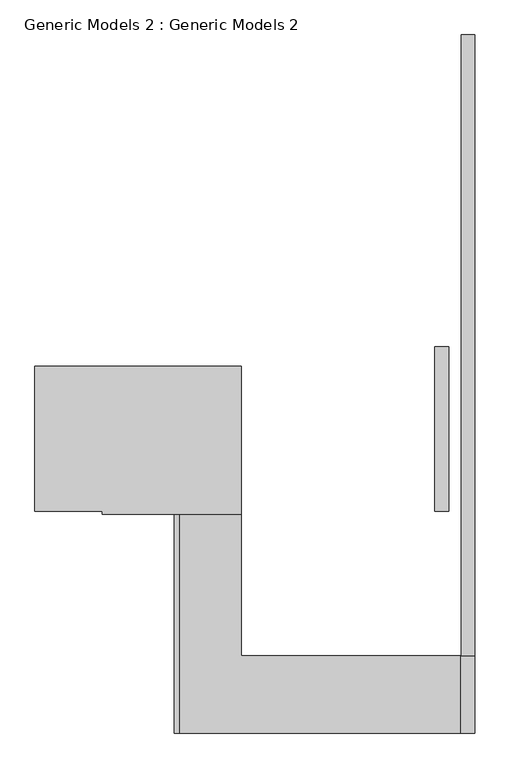
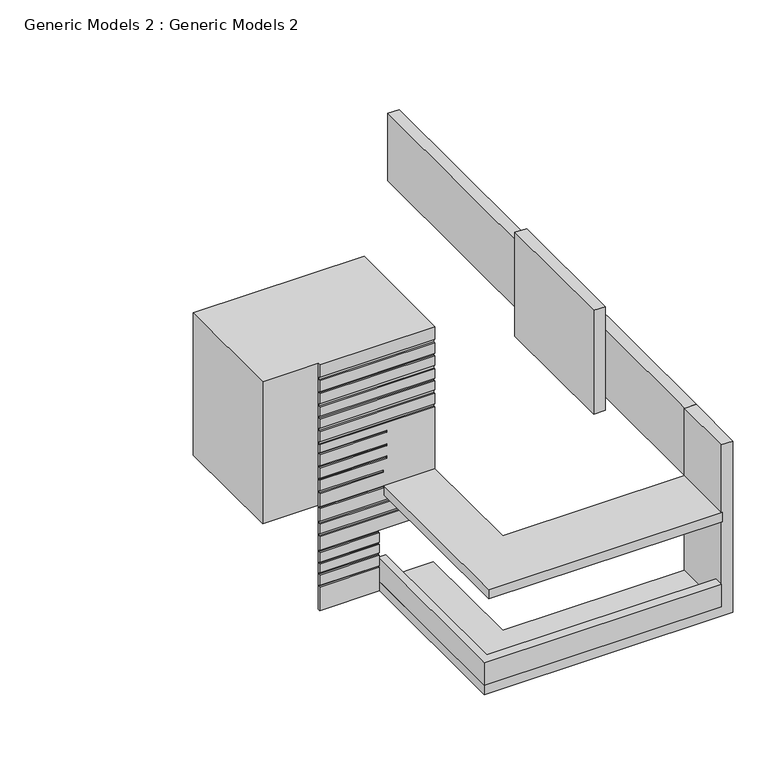
"""IFC4 building model written with IfcOpenShell, lengths in millimetres: proxy geometry, Generic Models 2 : Generic Models 2."""

from ifc_helpers import new_model, si_unit, frame, origin, place, context, project, spatial, polyline, outline, extrude, faceted_brep, source, transform, mapped, element, save


def generic_models_2_generic_models_2_8bbb9965(model_context):
    return source(origin(), model_context, "Body", "SolidModel", [
        extrude(outline(polyline([(-12215.152412, -15011.776778), (-12215.152412, -9476.6468404), (-10657.4321088, -9476.6468404), (-10657.4321088, -13058.0468404), (-5084.7494797, -13058.0468404), (-5084.7494797, -15011.776778), (-12215.152412, -15011.776778)])), frame((0.0, 0.0, 6096.0), z_axis=(0.0, 0.0, 1.0), x_axis=(1.0, 0.0, 0.0)), (0.0, 0.0, 1.0), 304.8),
        faceted_brep([(-15877.1321088, -9400.4468404, 6400.8), (-15877.1321088, -5738.2962979, 6400.8), (-10657.4321088, -5738.2962979, 6400.8), (-10657.4321088, -9400.4468404, 6400.8), (-14180.7645284, -9400.4468404, 6400.8), (-15877.1321088, -9400.4468404, 10988.8045332), (-14180.7645284, -9400.4468404, 10988.8045332), (-15877.1321088, -5738.2962979, 10988.8045332), (-10657.4321088, -5738.2962979, 10988.8045332), (-10657.4321088, -9476.6468404, 10988.8045332), (-14180.7645284, -9476.6468404, 10988.8045332), (-14180.7645284, -9476.6468404, 10585.2742098), (-10657.4321088, -9476.6468404, 10585.2742098), (-14180.7645284, -9476.6468404, 3048.0), (-12351.7136239, -9476.6468404, 3048.0), (-12351.7136239, -9476.6468404, 3808.1006121), (-14180.7645284, -9476.6468404, 3808.1006121), (-10657.4321088, -9476.6468404, 10470.2187496), (-14180.7645284, -9476.6468404, 10470.2187496), (-14180.7645284, -9476.6468404, 10122.5004137), (-10657.4321088, -9476.6468404, 10122.5004137), (-12351.7136239, -9476.6468404, 4611.1019692), (-12351.7136239, -9476.6468404, 4920.5427652), (-14180.7645284, -9476.6468404, 4920.5427652), (-14180.7645284, -9476.6468404, 4611.1019692), (-12351.7136239, -9476.6468404, 4276.4973082), (-12351.7136239, -9476.6468404, 4545.5762612), (-14180.7645284, -9476.6468404, 4545.5762612), (-14180.7645284, -9476.6468404, 4276.4973082), (-12351.7136239, -9476.6468404, 3862.9129914), (-12351.7136239, -9476.6468404, 4196.7702109), (-14180.7645284, -9476.6468404, 4196.7702109), (-14180.7645284, -9476.6468404, 3862.9129914), (-10657.4321088, -9476.6468404, 9733.5791761), (-10657.4321088, -9476.6468404, 10048.7503573), (-14180.7645284, -9476.6468404, 10048.7503573), (-14180.7645284, -9476.6468404, 9733.5791761), (-10657.4321088, -9476.6468404, 9327.208916), (-10657.4321088, -9476.6468404, 9618.9714739), (-14180.7645284, -9476.6468404, 9618.9714739), (-14180.7645284, -9476.6468404, 9327.208916), (-10657.4321088, -9476.6468404, 8943.2731135), (-10657.4321088, -9476.6468404, 9235.5227542), (-14180.7645284, -9476.6468404, 9235.5227542), (-14180.7645284, -9476.6468404, 8943.2731135), (-10657.4321088, -9476.6468404, 8496.3030748), (-10657.4321088, -9476.6468404, 8828.6654113), (-14180.7645284, -9476.6468404, 8828.6654113), (-14180.7645284, -9476.6468404, 8496.3030748), (-10657.4321088, -9476.6468404, 5929.0905449), (-10657.4321088, -9476.6468404, 8398.8865279), (-14180.7645284, -9476.6468404, 8398.8865279), (-14180.7645284, -9476.6468404, 8150.3954044), (-12128.9471301, -9476.6468404, 8150.3954044), (-12128.9471301, -9476.6468404, 8086.8954044), (-14180.7645284, -9476.6468404, 8086.8954044), (-14180.7645284, -9476.6468404, 7722.7010848), (-12128.9471301, -9476.6468404, 7722.7010848), (-12128.9471301, -9476.6468404, 7648.2060783), (-14180.7645284, -9476.6468404, 7648.2060783), (-14180.7645284, -9476.6468404, 7327.3045121), (-12128.9471301, -9476.6468404, 7327.3045121), (-12128.9471301, -9476.6468404, 7252.8095056), (-14180.7645284, -9476.6468404, 7252.8095056), (-14180.7645284, -9476.6468404, 6914.716784), (-12215.152412, -9476.6468404, 6914.716784), (-12215.152412, -9476.6468404, 6823.0306223), (-14180.7645284, -9476.6468404, 6823.0306223), (-14180.7645284, -9476.6468404, 6400.8), (-12215.152412, -9476.6468404, 6400.8), (-12215.152412, -9476.6468404, 6335.9478878), (-14180.7645284, -9476.6468404, 6335.9478878), (-14180.7645284, -9476.6468404, 5929.0905449), (-10657.4321088, -9476.6468404, 5527.9635871), (-10657.4321088, -9476.6468404, 5837.4043831), (-14180.7645284, -9476.6468404, 5837.4043831), (-14180.7645284, -9476.6468404, 5527.9635871), (-14180.7645284, -9476.6468404, 5004.8316632), (-10657.4321088, -9476.6468404, 5004.8316632), (-10657.4321088, -9476.6468404, 5430.5470402), (-14180.7645284, -9476.6468404, 5430.5470402), (-14180.7645284, -9400.4468404, 3048.0), (-14180.7645284, -9425.8468404, 3808.1006121), (-14180.7645284, -9425.8468404, 3862.9129914), (-14180.7645284, -9425.8468404, 4196.7702109), (-14180.7645284, -9425.8468404, 4276.4973082), (-14180.7645284, -9425.8468404, 4545.5762612), (-14180.7645284, -9425.8468404, 4611.1019692), (-14180.7645284, -9425.8468404, 4920.5427652), (-14180.7645284, -9425.8468404, 5004.8316632), (-14180.7645284, -9425.8468404, 5430.5470402), (-14180.7645284, -9425.8468404, 5527.9635871), (-14180.7645284, -9425.8468404, 5837.4043831), (-14180.7645284, -9425.8468404, 5929.0905449), (-14180.7645284, -9425.8468404, 6335.9478878), (-14180.7645284, -9425.8468404, 6400.8), (-14180.7645284, -9425.8468404, 6823.0306223), (-14180.7645284, -9425.8468404, 6914.716784), (-14180.7645284, -9425.8468404, 7252.8095056), (-14180.7645284, -9425.8468404, 7327.3045121), (-14180.7645284, -9425.8468404, 7648.2060783), (-14180.7645284, -9425.8468404, 7722.7010848), (-14180.7645284, -9425.8468404, 8086.8954044), (-14180.7645284, -9425.8468404, 8150.3954044), (-14180.7645284, -9425.8468404, 8398.8865279), (-14180.7645284, -9425.8468404, 8496.3030748), (-14180.7645284, -9425.8468404, 8828.6654113), (-14180.7645284, -9425.8468404, 8943.2731135), (-14180.7645284, -9425.8468404, 9235.5227542), (-14180.7645284, -9425.8468404, 9327.208916), (-14180.7645284, -9425.8468404, 9618.9714739), (-14180.7645284, -9425.8468404, 9733.5791761), (-14180.7645284, -9425.8468404, 10048.7503573), (-14180.7645284, -9425.8468404, 10122.5004137), (-14180.7645284, -9425.8468404, 10470.2187496), (-14180.7645284, -9425.8468404, 10585.2742098), (-10657.4321088, -9425.8468404, 10585.2742098), (-10657.4321088, -9425.8468404, 10470.2187496), (-10657.4321088, -9425.8468404, 10122.5004137), (-10657.4321088, -9425.8468404, 10048.7503573), (-10657.4321088, -9425.8468404, 9733.5791761), (-10657.4321088, -9425.8468404, 9618.9714739), (-10657.4321088, -9425.8468404, 9327.208916), (-10657.4321088, -9425.8468404, 9235.5227542), (-10657.4321088, -9425.8468404, 8943.2731135), (-10657.4321088, -9425.8468404, 8828.6654113), (-10657.4321088, -9425.8468404, 8496.3030748), (-10657.4321088, -9425.8468404, 8398.8865279), (-10657.4321088, -9425.8468404, 5929.0905449), (-10657.4321088, -9425.8468404, 5837.4043831), (-10657.4321088, -9425.8468404, 5527.9635871), (-10657.4321088, -9425.8468404, 5430.5470402), (-10657.4321088, -9400.4468404, 5004.8316632), (-12351.7136239, -9400.4468404, 5004.8316632), (-12351.7136239, -9400.4468404, 3048.0), (-12351.7136239, -9425.8468404, 5004.8316632), (-12351.7136239, -9425.8468404, 4920.5427652), (-12351.7136239, -9425.8468404, 4611.1019692), (-12351.7136239, -9425.8468404, 4545.5762612), (-12351.7136239, -9425.8468404, 4276.4973082), (-12351.7136239, -9425.8468404, 4196.7702109), (-12351.7136239, -9425.8468404, 3862.9129914), (-12351.7136239, -9425.8468404, 3808.1006121), (-12128.9471301, -9425.8468404, 8150.3954044), (-12128.9471301, -9425.8468404, 8086.8954044), (-12128.9471301, -9425.8468404, 7722.7010848), (-12128.9471301, -9425.8468404, 7648.2060783), (-12128.9471301, -9425.8468404, 7327.3045121), (-12128.9471301, -9425.8468404, 7252.8095056), (-12215.152412, -9425.8468404, 6914.716784), (-12215.152412, -9425.8468404, 6823.0306223), (-12215.152412, -9425.8468404, 6400.8), (-12215.152412, -9425.8468404, 6335.9478878)], [[[0, 1, 2, 3, 4]], [[5, 0, 4, 6]], [[7, 8, 2, 1]], [[5, 7, 1, 0]], [[9, 10, 11, 12]], [[13, 14, 15, 16]], [[17, 18, 19, 20]], [[21, 22, 23, 24]], [[25, 26, 27, 28]], [[29, 30, 31, 32]], [[33, 34, 35, 36]], [[37, 38, 39, 40]], [[41, 42, 43, 44]], [[45, 46, 47, 48]], [[49, 50, 51, 52, 53, 54, 55, 56, 57, 58, 59, 60, 61, 62, 63, 64, 65, 66, 67, 68, 69, 70, 71, 72]], [[73, 74, 75, 76]], [[77, 78, 79, 80]], [[10, 6, 4, 81, 13, 16, 82, 83, 32, 31, 84, 85, 28, 27, 86, 87, 24, 23, 88, 89, 77, 80, 90, 91, 76, 75, 92, 93, 72, 71, 94, 95, 68, 67, 96, 97, 64, 63, 98, 99, 60, 59, 100, 101, 56, 55, 102, 103, 52, 51, 104, 105, 48, 47, 106, 107, 44, 43, 108, 109, 40, 39, 110, 111, 36, 35, 112, 113, 19, 18, 114, 115, 11]], [[10, 9, 8, 7, 5, 6]], [[2, 8, 9, 12, 116, 117, 17, 20, 118, 119, 34, 33, 120, 121, 38, 37, 122, 123, 42, 41, 124, 125, 46, 45, 126, 127, 50, 49, 128, 129, 74, 73, 130, 131, 79, 78, 132, 3]], [[3, 132, 133, 134, 81, 4]], [[132, 78, 77, 89, 135, 133]], [[14, 13, 81, 134]], [[134, 133, 135, 136, 22, 21, 137, 138, 26, 25, 139, 140, 30, 29, 141, 142, 15, 14]], [[116, 115, 114, 117]], [[117, 114, 18, 17]], [[115, 116, 12, 11]], [[135, 89, 88, 136]], [[118, 113, 112, 119]], [[120, 111, 110, 121]], [[122, 109, 108, 123]], [[124, 107, 106, 125]], [[126, 105, 104, 127]], [[143, 103, 102, 144]], [[145, 101, 100, 146]], [[147, 99, 98, 148]], [[149, 97, 96, 150]], [[151, 95, 94, 152]], [[128, 93, 92, 129]], [[130, 91, 90, 131]], [[137, 87, 86, 138]], [[139, 85, 84, 140]], [[141, 83, 82, 142]], [[119, 112, 35, 34]], [[113, 118, 20, 19]], [[121, 110, 39, 38]], [[111, 120, 33, 36]], [[123, 108, 43, 42]], [[109, 122, 37, 40]], [[125, 106, 47, 46]], [[107, 124, 41, 44]], [[127, 104, 51, 50]], [[105, 126, 45, 48]], [[143, 144, 54, 53]], [[144, 102, 55, 54]], [[103, 143, 53, 52]], [[145, 146, 58, 57]], [[146, 100, 59, 58]], [[101, 145, 57, 56]], [[147, 148, 62, 61]], [[148, 98, 63, 62]], [[99, 147, 61, 60]], [[149, 150, 66, 65]], [[150, 96, 67, 66]], [[97, 149, 65, 64]], [[151, 152, 70, 69]], [[152, 94, 71, 70]], [[95, 151, 69, 68]], [[129, 92, 75, 74]], [[93, 128, 49, 72]], [[131, 90, 80, 79]], [[91, 130, 73, 76]], [[136, 88, 23, 22]], [[138, 86, 27, 26]], [[87, 137, 21, 24]], [[140, 84, 31, 30]], [[85, 139, 25, 28]], [[142, 82, 16, 15]], [[83, 141, 29, 32]]]),
        extrude(outline(polyline([(-5098.6527592, -13058.0468404), (-5098.6527592, 2639.1531596), (-4751.9321088, 2639.1531596), (-4751.9321088, -13058.0468404), (-5098.6527592, -13058.0468404)])), frame((0.0, 0.0, 6400.8), z_axis=(0.0, 0.0, 1.0), x_axis=(1.0, 0.0, 0.0)), (0.0, 0.0, 1.0), 2178.143726),
        extrude(outline(polyline([(-5417.9230491, -9400.4468404), (-5770.8398298, -9400.4468404), (-5770.8398298, -5247.5468404), (-5417.9230491, -5247.5468404), (-5417.9230491, -9400.4468404)])), frame((0.0, 0.0, 6400.8), z_axis=(0.0, 0.0, 1.0), x_axis=(1.0, 0.0, 0.0)), (0.0, 0.0, 1.0), 3351.6929741),
        extrude(outline(polyline([(-12351.7136239, -9400.4468404), (-12120.513383, -9400.4468404), (-12120.513383, -14738.7800298), (-5107.5321088, -14738.7800298), (-5107.5321088, -15011.776778), (-12351.7136239, -15011.776778), (-12351.7136239, -9400.4468404)])), frame((0.0, 0.0, 3352.8), z_axis=(0.0, 0.0, 1.0), x_axis=(1.0, 0.0, 0.0)), (0.0, 0.0, 1.0), 736.6),
        faceted_brep([(-12351.7136239, -15011.776778, 3048.0), (-12351.7136239, -15011.776778, 3352.8), (-12351.7136239, -9400.4468404, 3352.8), (-12351.7136239, -9400.4468404, 3048.0), (-10657.4321088, -9400.4468404, 3048.0), (-10657.4321088, -9400.4468404, 3352.8), (-10657.4321088, -13058.0468404, 3352.8), (-10657.4321088, -13058.0468404, 3048.0), (-4751.9321088, -15011.776778, 3048.0), (-4751.9321088, -15011.776778, 8578.943726), (-5107.5321088, -15011.776778, 8578.943726), (-5107.5321088, -15011.776778, 3352.8), (-5107.5321088, -13058.0468404, 3352.8), (-4751.9321088, -13058.0468404, 3048.0), (-5107.5321088, -13058.0468404, 8578.943726), (-4751.9321088, -13058.0468404, 8578.943726)], [[[0, 1, 2, 3]], [[4, 5, 6, 7]], [[1, 0, 8, 9, 10, 11]], [[2, 1, 11, 12, 6, 5]], [[3, 2, 5, 4]], [[0, 3, 4, 7, 13, 8]], [[13, 7, 6, 12, 14, 15]], [[9, 8, 13, 15]], [[10, 9, 15, 14]], [[11, 10, 14, 12]]]),
    ])


if __name__ == "__main__":
    model = new_model("IFC4")
    model_context = context("Model", 3, world=origin())
    ifc_project = project(units=[si_unit("LENGTHUNIT", "METRE", prefix="MILLI")], contexts=[model_context])
    site = spatial("IfcSite", under=ifc_project)
    building = spatial("IfcBuilding", under=site)
    placement = place(None, origin())
    generic_models_2_generic_models_2_shape = generic_models_2_generic_models_2_8bbb9965(model_context)
    element("IfcBuildingElementProxy", 1, Name="Generic Models 2 : Generic Models 2", ObjectType="Generic Models 2 : Generic Models 2", at=placement, inside=building, context=model_context, shape_type="MappedRepresentation", body=[
        mapped(generic_models_2_generic_models_2_shape, transform((0.0, 0.0, 0.0), x_axis=(1.0, 0.0, 0.0), y_axis=(0.0, 1.0, 0.0), z_axis=(0.0, 0.0, 1.0))),
    ])
    save(model, "model.ifc")
